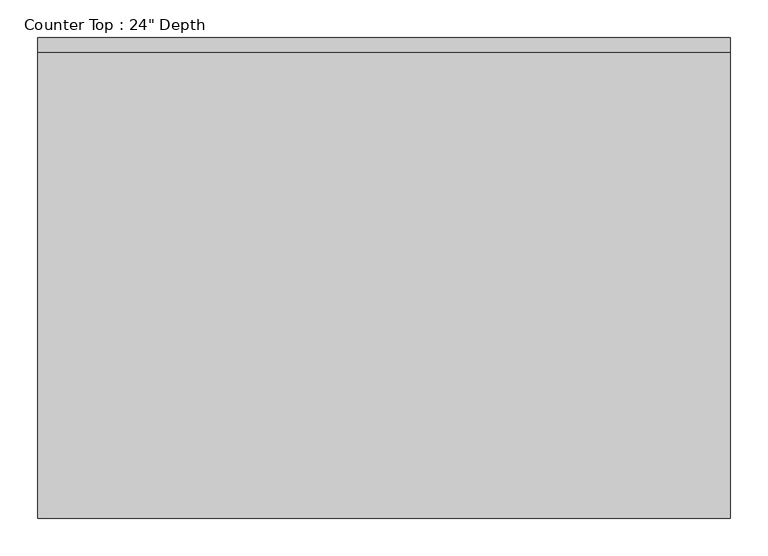
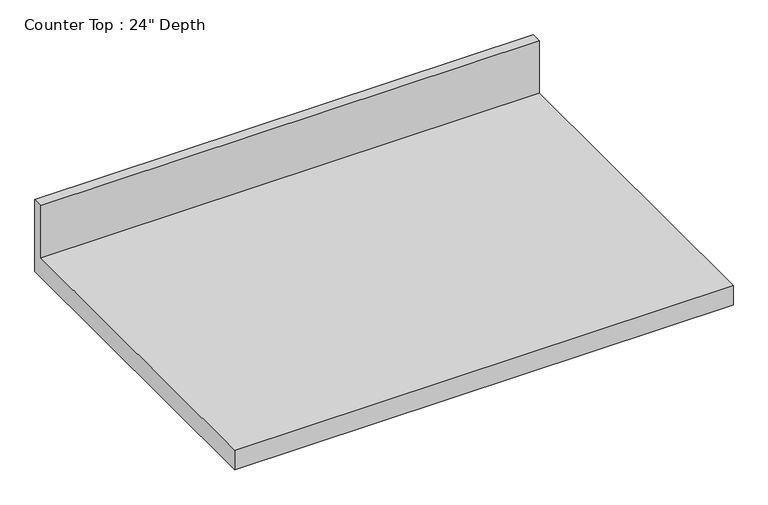
"""IFC4 building model written with IfcOpenShell, lengths in millimetres: furniture geometry."""

from ifc_helpers import new_model, si_unit, frame, origin, place, context, project, spatial, polyline, outline, extrude, source, transform, mapped, element, save


def furniture_4e2f607e(model_context):
    return source(origin(), model_context, "Body", "SweptSolid", [
        extrude(outline(polyline([(0.0, 1016.0), (0.0, 876.3), (-635.0, 876.3), (-635.0, 914.4), (-19.05, 914.4), (-19.05, 1016.0), (0.0, 1016.0)])), frame((-1200.4622951, 0.0, 0.0), z_axis=(1.0, 0.0, 0.0), x_axis=(0.0, 1.0, 0.0)), (0.0, 0.0, 1.0), 914.4),
    ])


if __name__ == "__main__":
    model = new_model("IFC4")
    model_context = context("Model", 3, world=origin())
    ifc_project = project(units=[si_unit("LENGTHUNIT", "METRE", prefix="MILLI")], contexts=[model_context])
    site = spatial("IfcSite", under=ifc_project)
    building = spatial("IfcBuilding", under=site)
    placement = place(None, origin())
    furniture_shape = furniture_4e2f607e(model_context)
    element("IfcFurniture", 1, ObjectType="Counter Top : 24\" Depth", at=placement, inside=building, context=model_context, shape_type="MappedRepresentation", body=[
        mapped(furniture_shape, transform((0.0, 0.0, 0.0), x_axis=(1.0, 0.0, 0.0), y_axis=(0.0, 1.0, 0.0), z_axis=(0.0, 0.0, 1.0))),
    ])
    save(model, "model.ifc")

# Revit data of these elements
# Type "Counter Top : 24\" Depth"
#   Assembly Code = "C1030400"
#   Counter Thickness = 0' - 1 1/2"
#   Depth = 2' - 1"
#   Height = 3' - 0"
#   Length [instance default] = 8' - 0"
#   Counter Top Material = none
#   Default Elevation = 0
# Element 1 (IfcFurniture, "Counter Top : 24\" Depth")
#   Length = 3' - 0"
#   Materials on its faces: "Counter Top"
# Materials
#   "Counter Top": class "Wood", colour RGB 226 177 128, transparency 0
